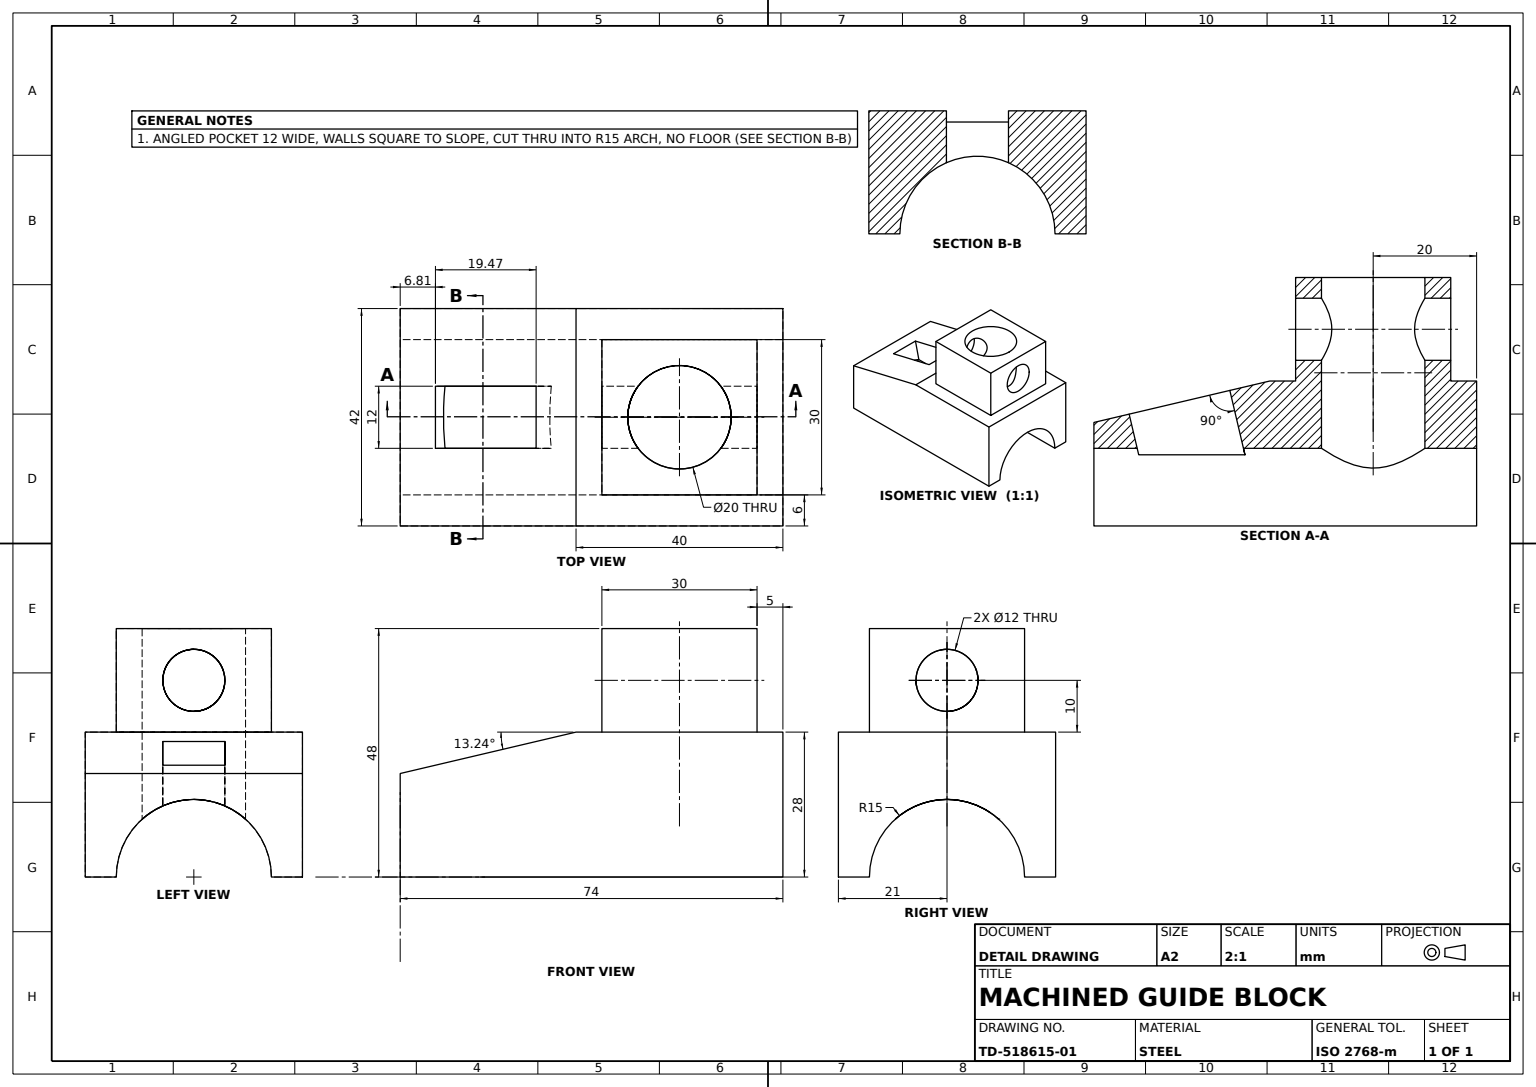
SolidWorks part; units mm, degrees
material "Plain Carbon Steel"
ref_plane "Front Plane" through (0, 0, 0) normal (0, 0, 1) x (1, 0, 0)
ref_plane "Top Plane" through (0, 0, 0) normal (0, 1, 0) x (1, 0, 0)
ref_plane "Right Plane" through (0, 0, 0) normal (1, 0, 0) x (0, 0, -1)
sketch "Base Block Profile Sketch" plane through (0, 0, 0) normal (0, 0, 1) x (1, 0, 0)
  line L0 (0, 0) -> (74, 0)
  line L1 (74, 0) -> (74, 28)
  line L2 (74, 28) -> (34, 28)
  line L3 (34, 28) -> (0, 20)
  line L4 (0, 20) -> (0, 0)
  dimension "D1" = 28
  dimension "D2" = 74
  dimension "D3" = 20
  dimension "D4" = 40
extrude "Base Block" add sketch "Base Block Profile Sketch" along normal blind 42
sketch "Top Boss Sketch" plane through (0, 28, 0) normal (0, 1, 0) x (1, 0, 0)
  line L0 (74, -42) -> (34, -42) construction
  line L1 (39, -6) -> (69, -6)
  line L2 (39, -6) -> (39, -36)
  line L3 (39, -36) -> (69, -36)
  line L4 (69, -6) -> (69, -36)
  line L5 (34, -42) -> (34, 0) construction
  dimension "D1" = 30
  dimension "D2" = 30
  dimension "D3" = 6
  dimension "D4" = 5
extrude "Top Boss 30x30" add sketch "Top Boss Sketch" along normal blind 20
sketch "Vertical Bore Sketch" plane through (0, 48, 0) normal (0, 1, 0) x (1, 0, 0)
  line L0 (54, -6) -> (54, -36) construction
  line L1 (69, -6) -> (39, -6) construction
  line L2 (39, -36) -> (69, -36) construction
  circle A0 centre (54, -21) radius 10
  dimension "D1" = 20
extrude "Vertical Bore" cut sketch "Vertical Bore Sketch" against normal through all
sketch "Cross Hole Sketch" plane through (39, 0, 0) normal (-1, 0, 0) x (0, 0, 1)
  line L0 (21, 48) -> (21, 28) construction
  line L1 (6, 48) -> (36, 48) construction
  line L2 (42, 28) -> (0, 28) construction
  circle A0 centre (21, 38) radius 6
  dimension "D1" = 12
extrude "Cross Hole" cut sketch "Cross Hole Sketch" against normal through all
sketch "Angled Pocket Sketch" plane through (-4.459, 18.9508, 0) normal (-0.229, 0.9734, 0) x (0.9734, 0.229, 0)
  line L0 (39.5093, -21) -> (4.5808, -21) construction
  line L1 (39.5093, -42) -> (39.5093, 0) construction
  line L2 (4.5808, -42) -> (4.5808, 0) construction
  line L3 (11.5808, -21) -> (11.5808, -15)
  line L4 (11.5808, -15) -> (31.5808, -15)
  line L5 (31.5808, -15) -> (31.5808, -27)
  line L6 (31.5808, -27) -> (11.5808, -27)
  line L7 (11.5808, -27) -> (11.5808, -21)
  dimension "D1" = 6
  dimension "D2" = 6
  dimension "D3" = 20
  dimension "D4" = 7
extrude "Angled Pocket" cut sketch "Angled Pocket Sketch" against normal through all
sketch "Arch Cutout Sketch" plane through (0, 0, 0) normal (-1, 0, 0) x (0, 0, 1)
  line L0 (21, 20) -> (21, 0) construction
  line L1 (42, 20) -> (0, 20) construction
  line L2 (42, 0) -> (0, 0) construction
  line L3 (6, 0) -> (36, 0) construction
  arc A0 (36, 0) -> (6, 0) centre (21, 0) ccw
  dimension "D1" = 30
extrude "Arch Cutout" cut sketch "Arch Cutout Sketch" along normal through all and the other way through all
